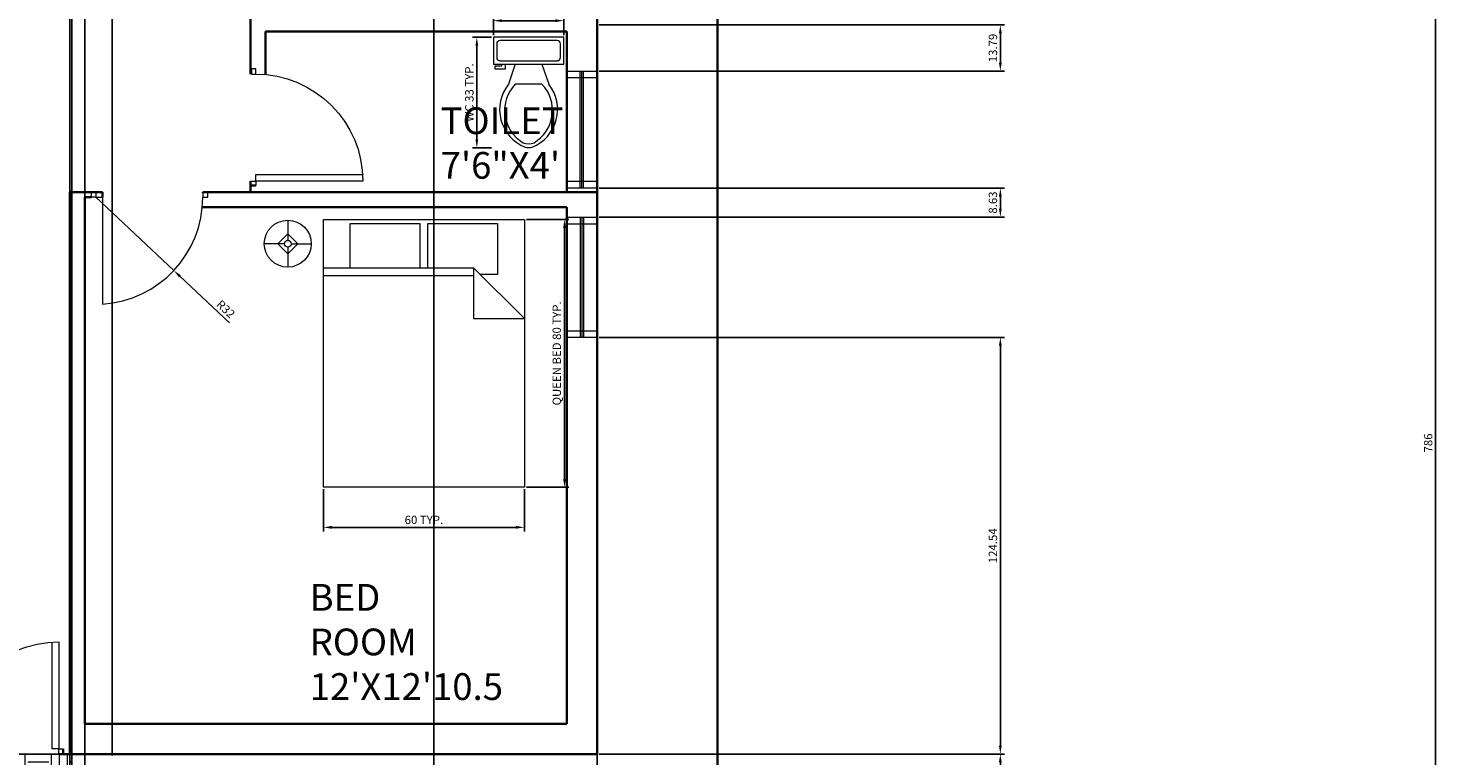
# Model space of a CAD drawing. Units: inches. Extents: x 204 to 942, y 1794 to 2670.
# Tile 5 of 6: x 521 to 942, y 2138 to 2355. Entities that reach past the tile are written whole.
import ezdxf

# ---------------------------------------------------------------- set-up
doc = ezdxf.new("R2010")
doc.units = ezdxf.units.IN
for name, color, linetype, lineweight in [('A-ANNO-DIMS', 2, 'Continuous', 18), ('A-AREA-IDEN', 7, 'Continuous', 18), ('A-DOOR', 3, 'Continuous', 18), ('A-FLOR-FIXT', 9, 'Continuous', 18), ('A-FLOR-OTLN', 7, 'Continuous', 25), ('A-FLOR-STRS', 7, 'Continuous', 25), ('A-FURN', 8, 'Continuous', 18), ('A-GLAZ', 4, 'Continuous', 18), ('A-WALL', 7, 'Continuous', 35), ('C-PROP', 7, 'Continuous', 35)]:
    doc.layers.add(name, color=color, linetype=linetype, lineweight=lineweight)
doc.layers.add('A-FLOR-PATT', color=251, linetype='Continuous', lineweight=13, true_color=0x636466)
doc.styles.get("Standard").update_dxf_attribs({"font": 'arial.ttf'})
doc.dimstyles.new('ISO-25', dxfattribs={"dimtxt": 2.5, "dimasz": 2.5, "dimexe": 1.25, "dimexo": 0.625, "dimtad": 1, "dimtxsty": 'Standard', "dimcen": 2.5, "dimadec": 0, "dimazin": 0, "dimtfac": 1, "dimtmove": 0, "dimatfit": 3, "dimfxl": 1, "dimarcsym": 0})

# ---------------------------------------------------------------- blocks, each defined once
blk = doc.blocks.new('Bed - Queen')
for p, q in [((0, -80.00003), (0, 0)), ((0, 0), (59.99999, 0)), ((59.99999, 0), (59.99999, -80.00003)), ((7.99999, -1.2), (28.79998, -1.2)), ((7.99999, -14.4), (7.99999, -1.2)), ((28.79998, -1.2), (28.79998, -14.4)), ((31.19999, -1.2), (51.99999, -1.2)), ((31.19999, -14.4), (31.19999, -1.2)), ((51.99999, -1.2), (51.99999, -16.4)), ((0, -14.4), (44.8, -14.4)), ((44.8, -16.8), (0, -16.8)), ((59.99999, -29.6), (44.8, -14.4)), ((44.8, -14.4), (44.8, -29.6)), ((51.99999, -16.4), (46.79936, -16.4)), ((44.8, -29.6), (59.99999, -29.6)), ((59.99999, -80.00003), (0, -80.00003))]:
    blk.add_line(p, q)
blk = doc.blocks.new('Lamp - Table')
for p, q in [((0, 7), (0, 1)), ((-1, 0), (-7, 0)), ((0, 3), (-3, 0)), ((-3, 0), (0, -3)), ((3, 0), (0, 3)), ((0, -3), (3, 0)), ((1, 0), (7, 0)), ((0, -1), (0, -7))]:
    blk.add_line(p, q)
for radius in [7, 1]:
    blk.add_circle((0, 0), radius)
blk = doc.blocks.new('Toilet - top')
for p, q in [((9.5, -6), (9.5, -2)), ((-8, -8.5), (-8, -8)), ((-7, -8), (-7, -9.5)), ((-4, -8), (-6, -14)), ((4, -8), (6, -14)), ((-10, -8.5), (-8, -8.5)), ((-10, -9.5), (-10, -8.5)), ((-7, -9.5), (-10, -9.5)), ((4, -14), (-4, -14))]:
    blk.add_line(p, q)
blk.add_lwpolyline([(10.5, -8), (10.5, 0), (-10.5, 0), (-10.5, -8)], close=True)
for points in [[(-9.5, -2), (-9.5, -6)], [(8.5, -1), (-8.5, -1)], [(-8.5, -7), (8.5, -7)]]:
    blk.add_lwpolyline(points)
for centre, radius, start, end in [((-8.62, -1.88), 0.884, 81.8699, 188.1301), ((8.62, -1.88), 0.884, 351.8699, 98.1301), ((-8.62, -6.12), 0.884, 171.8699, 278.1301), ((8.62, -6.12), 0.884, 261.8699, 8.1301), ((3.52, -21.58), 12.17, 141.4691, 247.9714), ((4.2, -21.82), 11.33, 136.3677, 238.9468), ((-3.52, -21.58), 12.17, 292.0284, 38.5307), ((-4.2, -21.82), 11.33, 301.053, 43.6321), ((0, -27.88), 4, 245.7318, 294.2682), ((0, -29), 4, 254.8605, 285.1395)]:
    blk.add_arc(centre, radius, start, end)
blk = doc.blocks.new('*D12')
at = {"layer": 'A-ANNO-DIMS', "color": 0, "lineweight": -2, "transparency": 16777216}
for p, q in [((727.37, 2624.26), (942.46, 2624.26)), ((941.21, 2621.76), (941.21, 1840.76)), ((727.37, 1838.26), (942.46, 1838.26))]:
    blk.add_line(p, q, dxfattribs=at)
at = {"layer": 'A-ANNO-DIMS', "color": 0, "transparency": 16777216}
for points in [[(940.79, 2621.76), (941.63, 2621.76), (941.21, 2624.26)], [(940.79, 1840.76), (941.63, 1840.76), (941.21, 1838.26)]]:
    blk.add_solid(points, dxfattribs=at)
at = {"layer": 'Defpoints', "color": 0, "transparency": 16777216}
for p in [(726.74, 2624.26), (726.74, 1838.26), (941.21, 1838.26)]:
    blk.add_point(p, dxfattribs=at)
at = {"layer": 'A-ANNO-DIMS', "color": 0, "transparency": 16777216, "insert": (939.31, 2231.26), "char_height": 2.5, "attachment_point": 5, "rotation": 90}
blk.add_mtext('786', dxfattribs=at)
blk = doc.blocks.new('WIN-36IN')
for p, q in [((0, 9), (36, 9)), ((0, 0), (0, 9)), ((2, 0), (2, 9)), ((34, 0), (34, 9)), ((36, 9), (36, 0)), ((0, 5), (36, 5)), ((0, 4.5), (36, 4.5)), ((0, 4), (36, 4)), ((36, 0), (0, 0)), ((0, 0), (2, 0)), ((36, 0), (34, 0))]:
    blk.add_line(p, q)
blk = doc.blocks.new('WIN-35IN')
for p, q in [((0, 0), (0, 35)), ((0, 35), (9, 35)), ((4, 0), (4, 35)), ((4.5, 0), (4.5, 35)), ((5, 0), (5, 35)), ((9, 35), (9, 0)), ((9, 35), (9, 33)), ((9, 33), (0, 33)), ((9, 2), (0, 2)), ((9, 0), (0, 0)), ((9, 0), (9, 2))]:
    blk.add_line(p, q)
blk = doc.blocks.new('DOOR-SWING-32IN')
for p, q in [((3.26, 1.55), (3.26, 33.49)), ((1.26, 1.55), (3.26, 1.55))]:
    blk.add_line(p, q)
blk.add_lwpolyline([(1.26, 33.55), (1.26, 1.55), (3.26, 1.55)])
for points in [[(1.26, 1.55), (0, 1.55), (0, 0), (1.26, 0)], [(33.26, 1.55), (34.79, 1.55), (34.79, 0.26), (33.26, 0.26)]]:
    blk.add_lwpolyline(points, close=True)
blk.add_arc((1.26, 1.55), 32, 0, 90)
blk = doc.blocks.new('*D22')
at = {"layer": 'A-ANNO-DIMS', "color": 0, "lineweight": -2, "transparency": 16777216}
for p, q in [((669.66, 2298.04), (682.29, 2298.04)), ((681.04, 2220.54), (681.04, 2295.54)), ((669.66, 2218.04), (682.29, 2218.04))]:
    blk.add_line(p, q, dxfattribs=at)
at = {"layer": 'A-ANNO-DIMS', "color": 0, "transparency": 16777216}
for points in [[(680.62, 2295.54), (681.46, 2295.54), (681.04, 2298.04)], [(680.62, 2220.54), (681.46, 2220.54), (681.04, 2218.04)]]:
    blk.add_solid(points, dxfattribs=at)
at = {"layer": 'Defpoints', "color": 0, "transparency": 16777216}
for p in [(669.04, 2298.04), (681.04, 2298.04), (669.04, 2218.04)]:
    blk.add_point(p, dxfattribs=at)
at = {"layer": 'A-ANNO-DIMS', "color": 0, "transparency": 16777216, "insert": (679.05, 2258.04), "char_height": 2.5, "attachment_point": 5, "rotation": 90}
blk.add_mtext('QUEEN BED 80 TYP.', dxfattribs=at)
blk = doc.blocks.new('*D23')
at = {"layer": 'A-ANNO-DIMS', "color": 0, "lineweight": -2, "transparency": 16777216}
for p, q in [((609.04, 2217.41), (609.04, 2204.79)), ((669.04, 2217.41), (669.04, 2204.79)), ((611.54, 2206.04), (666.54, 2206.04))]:
    blk.add_line(p, q, dxfattribs=at)
at = {"layer": 'A-ANNO-DIMS', "color": 0, "transparency": 16777216}
for points in [[(611.54, 2206.46), (611.54, 2205.62), (609.04, 2206.04)], [(666.54, 2206.46), (666.54, 2205.62), (669.04, 2206.04)]]:
    blk.add_solid(points, dxfattribs=at)
at = {"layer": 'Defpoints', "color": 0, "transparency": 16777216}
for p in [(609.04, 2218.04), (669.04, 2218.04), (669.04, 2206.04)]:
    blk.add_point(p, dxfattribs=at)
at = {"layer": 'A-ANNO-DIMS', "color": 0, "transparency": 16777216, "insert": (639.04, 2207.94), "char_height": 2.5, "attachment_point": 5}
blk.add_mtext('60 TYP.', dxfattribs=at)
blk = doc.blocks.new('*D26')
at = {"layer": 'A-ANNO-DIMS', "color": 0, "lineweight": -2, "transparency": 16777216}
for p, q in [((659.18, 2352.53), (653.6, 2352.53)), ((654.85, 2321.99), (654.85, 2350.03)), ((659.18, 2319.49), (653.6, 2319.49))]:
    blk.add_line(p, q, dxfattribs=at)
at = {"layer": 'A-ANNO-DIMS', "color": 0, "transparency": 16777216}
for points in [[(654.43, 2350.03), (655.26, 2350.03), (654.85, 2352.53)], [(654.43, 2321.99), (655.26, 2321.99), (654.85, 2319.49)]]:
    blk.add_solid(points, dxfattribs=at)
at = {"layer": 'Defpoints', "color": 0, "transparency": 16777216}
for p in [(654.85, 2352.53), (659.8, 2352.53), (659.8, 2319.49)]:
    blk.add_point(p, dxfattribs=at)
at = {"layer": 'A-ANNO-DIMS', "color": 0, "transparency": 16777216, "insert": (652.93, 2336.01), "char_height": 2.5, "attachment_point": 5, "rotation": 90}
blk.add_mtext('WC 33 TYP.', dxfattribs=at)
blk = doc.blocks.new('*D27')
at = {"layer": 'A-ANNO-DIMS', "color": 0, "lineweight": -2, "transparency": 16777216}
for p, q in [((659.8, 2353.16), (659.8, 2358.74)), ((662.3, 2357.49), (678.3, 2357.49)), ((680.8, 2353.16), (680.8, 2358.74))]:
    blk.add_line(p, q, dxfattribs=at)
at = {"layer": 'A-ANNO-DIMS', "color": 0, "transparency": 16777216}
for points in [[(662.3, 2357.91), (662.3, 2357.07), (659.8, 2357.49)], [(678.3, 2357.91), (678.3, 2357.07), (680.8, 2357.49)]]:
    blk.add_solid(points, dxfattribs=at)
at = {"layer": 'Defpoints', "color": 0, "transparency": 16777216}
for p in [(680.8, 2357.49), (659.8, 2352.53), (680.8, 2352.53)]:
    blk.add_point(p, dxfattribs=at)
at = {"layer": 'A-ANNO-DIMS', "color": 0, "transparency": 16777216, "insert": (670.3, 2359.37), "char_height": 2.5, "attachment_point": 5}
blk.add_mtext('21 TYP.', dxfattribs=at)
blk = doc.blocks.new('*D45')
at = {"layer": 'A-ANNO-DIMS', "color": 0, "lineweight": -2, "transparency": 16777216}
for p, q in [((691.37, 2138.26), (812.46, 2138.26)), ((811.21, 2016.68), (811.21, 2135.76)), ((691.37, 2014.18), (812.46, 2014.18))]:
    blk.add_line(p, q, dxfattribs=at)
at = {"layer": 'A-ANNO-DIMS', "color": 0, "transparency": 16777216}
for points in [[(810.79, 2135.76), (811.62, 2135.76), (811.21, 2138.26)], [(810.79, 2016.68), (811.62, 2016.68), (811.21, 2014.18)]]:
    blk.add_solid(points, dxfattribs=at)
at = {"layer": 'Defpoints', "color": 0, "transparency": 16777216}
for p in [(690.74, 2138.26), (811.21, 2138.26), (690.74, 2014.18)]:
    blk.add_point(p, dxfattribs=at)
at = {"layer": 'A-ANNO-DIMS', "color": 0, "transparency": 16777216, "insert": (809.31, 2076.22), "char_height": 2.5, "attachment_point": 5, "rotation": 90}
blk.add_mtext('124.08', dxfattribs=at)
blk = doc.blocks.new('*D47')
at = {"layer": 'A-ANNO-DIMS', "color": 0, "lineweight": -2, "transparency": 16777216}
for p, q in [((533.86, 2137.88), (533.86, 2668.11)), ((536.36, 2666.86), (543.38, 2666.86)), ((545.88, 2137.88), (545.88, 2668.11))]:
    blk.add_line(p, q, dxfattribs=at)
at = {"layer": 'A-ANNO-DIMS', "color": 0, "transparency": 16777216}
for points in [[(536.36, 2667.28), (536.36, 2666.44), (533.86, 2666.86)], [(543.38, 2667.28), (543.38, 2666.44), (545.88, 2666.86)]]:
    blk.add_solid(points, dxfattribs=at)
at = {"layer": 'Defpoints', "color": 0, "transparency": 16777216}
for p in [(545.88, 2666.86), (533.86, 2137.26), (545.88, 2137.26)]:
    blk.add_point(p, dxfattribs=at)
at = {"layer": 'A-ANNO-DIMS', "color": 0, "transparency": 16777216, "insert": (539.87, 2668.76), "char_height": 2.5, "attachment_point": 5}
blk.add_mtext('12.012', dxfattribs=at)
blk = doc.blocks.new('*D48')
at = {"layer": 'A-ANNO-DIMS', "color": 0, "lineweight": -2, "transparency": 16777216}
for p, q in [((641.98, 2014.8), (641.98, 2668.11)), ((644.48, 2666.86), (688.24, 2666.86)), ((690.74, 2014.8), (690.74, 2668.11))]:
    blk.add_line(p, q, dxfattribs=at)
at = {"layer": 'A-ANNO-DIMS', "color": 0, "transparency": 16777216}
for points in [[(644.48, 2667.28), (644.48, 2666.44), (641.98, 2666.86)], [(688.24, 2667.28), (688.24, 2666.44), (690.74, 2666.86)]]:
    blk.add_solid(points, dxfattribs=at)
at = {"layer": 'Defpoints', "color": 0, "transparency": 16777216}
for p in [(690.74, 2666.86), (641.98, 2014.18), (690.74, 2014.18)]:
    blk.add_point(p, dxfattribs=at)
at = {"layer": 'A-ANNO-DIMS', "color": 0, "transparency": 16777216, "insert": (666.36, 2668.76), "char_height": 2.5, "attachment_point": 5}
blk.add_mtext('48.77', dxfattribs=at)
blk = doc.blocks.new('*D50')
at = {"layer": 'A-ANNO-DIMS', "color": 0, "lineweight": -2, "transparency": 16777216}
for p, q in [((533.24, 2587.63), (533.24, 1794.41)), ((537.74, 2578.63), (537.74, 1794.41)), ((530.74, 1795.66), (528.24, 1795.66)), ((533.24, 1795.66), (537.74, 1795.66)), ((540.24, 1795.66), (548.67, 1795.66))]:
    blk.add_line(p, q, dxfattribs=at)
at = {"layer": 'A-ANNO-DIMS', "color": 0, "transparency": 16777216}
for points in [[(530.74, 1796.08), (530.74, 1795.24), (533.24, 1795.66)], [(540.24, 1796.08), (540.24, 1795.24), (537.74, 1795.66)]]:
    blk.add_solid(points, dxfattribs=at)
at = {"layer": 'Defpoints', "color": 0, "transparency": 16777216}
for p in [(533.24, 2588.26), (537.74, 2579.26), (537.74, 1795.66)]:
    blk.add_point(p, dxfattribs=at)
at = {"layer": 'A-ANNO-DIMS', "color": 0, "transparency": 16777216, "insert": (545.7, 1797.56), "char_height": 2.5, "attachment_point": 5}
blk.add_mtext('4.5', dxfattribs=at)
blk = doc.blocks.new('*D60')
at = {"layer": 'A-ANNO-DIMS', "color": 0, "lineweight": -2, "transparency": 16777216}
for p, q in [((691.38, 2262.8), (812.46, 2262.8)), ((811.21, 2140.76), (811.21, 2260.3)), ((691.37, 2138.26), (812.46, 2138.26))]:
    blk.add_line(p, q, dxfattribs=at)
at = {"layer": 'A-ANNO-DIMS', "color": 0, "transparency": 16777216}
for points in [[(810.79, 2260.3), (811.62, 2260.3), (811.21, 2262.8)], [(810.79, 2140.76), (811.62, 2140.76), (811.21, 2138.26)]]:
    blk.add_solid(points, dxfattribs=at)
at = {"layer": 'Defpoints', "color": 0, "transparency": 16777216}
for p in [(690.76, 2262.8), (811.21, 2262.8), (690.74, 2138.26)]:
    blk.add_point(p, dxfattribs=at)
at = {"layer": 'A-ANNO-DIMS', "color": 0, "transparency": 16777216, "insert": (809.31, 2200.53), "char_height": 2.5, "attachment_point": 5, "rotation": 90}
blk.add_mtext('124.54', dxfattribs=at)
blk = doc.blocks.new('*D61')
at = {"layer": 'A-ANNO-DIMS', "color": 0, "lineweight": -2, "transparency": 16777216}
for p, q in [((691.38, 2356.22), (812.46, 2356.22)), ((811.21, 2344.93), (811.21, 2353.72)), ((691.38, 2342.43), (812.46, 2342.43))]:
    blk.add_line(p, q, dxfattribs=at)
at = {"layer": 'A-ANNO-DIMS', "color": 0, "transparency": 16777216}
for points in [[(810.79, 2353.72), (811.62, 2353.72), (811.21, 2356.22)], [(810.79, 2344.93), (811.62, 2344.93), (811.21, 2342.43)]]:
    blk.add_solid(points, dxfattribs=at)
at = {"layer": 'Defpoints', "color": 0, "transparency": 16777216}
for p in [(690.76, 2356.22), (811.21, 2356.22), (690.75, 2342.43)]:
    blk.add_point(p, dxfattribs=at)
at = {"layer": 'A-ANNO-DIMS', "color": 0, "transparency": 16777216, "insert": (809.31, 2349.33), "char_height": 2.5, "attachment_point": 5, "rotation": 90}
blk.add_mtext('13.79', dxfattribs=at)
blk = doc.blocks.new('*D62')
at = {"layer": 'A-ANNO-DIMS', "color": 0, "lineweight": -2, "transparency": 16777216}
for p, q in [((691.38, 2307.43), (812.46, 2307.43)), ((811.21, 2301.3), (811.21, 2304.93)), ((691.38, 2298.8), (812.46, 2298.8))]:
    blk.add_line(p, q, dxfattribs=at)
at = {"layer": 'A-ANNO-DIMS', "color": 0, "transparency": 16777216}
for points in [[(810.79, 2304.93), (811.62, 2304.93), (811.21, 2307.43)], [(810.79, 2301.3), (811.62, 2301.3), (811.21, 2298.8)]]:
    blk.add_solid(points, dxfattribs=at)
at = {"layer": 'Defpoints', "color": 0, "transparency": 16777216}
for p in [(690.75, 2307.43), (811.21, 2307.43), (690.76, 2298.8)]:
    blk.add_point(p, dxfattribs=at)
at = {"layer": 'A-ANNO-DIMS', "color": 0, "transparency": 16777216, "insert": (809.31, 2303.12), "char_height": 2.5, "attachment_point": 5, "rotation": 90}
blk.add_mtext('8.63', dxfattribs=at)
blk = doc.blocks.new('*D63')
at = {"layer": 'A-ANNO-DIMS', "color": 0, "lineweight": -2, "transparency": 16777216}
for p, q in [((541.01, 2304.71), (564.33, 2282.8)), ((580.95, 2267.19), (566.15, 2281.09))]:
    blk.add_line(p, q, dxfattribs=at)
at = {"layer": 'A-ANNO-DIMS', "color": 0, "transparency": 16777216}
blk.add_solid([(566.44, 2281.39), (565.87, 2280.78), (564.33, 2282.8)], dxfattribs=at)
at = {"layer": 'Defpoints', "color": 0, "transparency": 16777216}
for p in [(541.01, 2304.71), (564.33, 2282.8)]:
    blk.add_point(p, dxfattribs=at)
at = {"layer": 'A-ANNO-DIMS', "color": 0, "transparency": 16777216, "insert": (579.63, 2271.04), "char_height": 2.5, "attachment_point": 5, "rotation": 316.7911}
blk.add_mtext('R32', dxfattribs=at)

msp = doc.modelspace()

# ---------------------------------------------------------------- hatches: boundary and pattern name
at = {"layer": 'A-FLOR-PATT'}
h = msp.add_hatch(dxfattribs=at)
h.set_pattern_fill('EARTH', color=256)
h.paths.add_polyline_path([(533.8633, 2137.2597), (533.8633, 2138.2597), (473.5284, 2138.2597), (473.5284, 2138.2472), (471.5284, 2138.2472), (437.5284, 2138.2472), (372.7443, 2138.2597), (336.7443, 2138.2597), (336.7443, 2014.1774), (533.8633, 2014.1774)])

# ---------------------------------------------------------------- linework, layer by layer
at = {"layer": 'A-DOOR'}
for p, q in [((541.0064, 2304.7082), (543.0064, 2304.7082)), ((543.0064, 2304.7082), (543.0064, 2272.7707))]:
    msp.add_line(p, q, dxfattribs=at)
for points in [[(541.0064, 2304.7082), (539.7443, 2304.7082), (539.7443, 2306.2597), (541.0064, 2306.2597)], [(573.0064, 2304.7082), (574.53, 2304.7082), (574.53, 2306.0038), (573.0064, 2306.0038)]]:
    msp.add_lwpolyline(points, close=True, dxfattribs=at)
msp.add_lwpolyline([(541.0064, 2304.7082), (543.0064, 2304.7082)], dxfattribs=at)
msp.add_arc((541.0064, 2304.7082), 32, 273.583322, 0, dxfattribs=at)
at = {"layer": 'A-FLOR-OTLN'}
msp.add_lwpolyline([(372.7443, 2588.2597), (690.7443, 2588.2597), (690.7443, 2138.2597), (372.7443, 2138.2597)], close=True, dxfattribs=at)
at = {"layer": 'A-FLOR-STRS'}
for p, q in [((533.8633, 2014.1774), (533.8633, 2138.2597)), ((641.9756, 2014.1774), (641.9756, 2138.2597)), ((690.7443, 2138.2597), (690.7443, 2014.1774))]:
    msp.add_line(p, q, dxfattribs=at)
at = {"layer": 'A-WALL'}
for p, q in [((690.7443, 2411.2597), (690.7443, 2330.2597)), ((587.2443, 2341.4841), (587.2443, 2358.7597)), ((681.7443, 2354.2597), (591.7443, 2354.2597)), ((591.7443, 2341.3856), (591.7443, 2354.2597)), ((681.7443, 2354.2597), (681.7443, 2306.2597)), ((690.7443, 2354.2597), (690.7443, 2301.7597)), ((533.2443, 2147.2597), (533.2443, 2306.2597)), ((537.7443, 2306.2597), (533.2443, 2306.2597)), ((537.7443, 2306.2597), (541.0064, 2306.2597)), ((537.7443, 2306.2597), (539.7443, 2306.2597)), ((541.0064, 2306.2597), (543.0064, 2306.2597)), ((543.0064, 2306.2597), (543.0064, 2304.7082)), ((573.0064, 2306.2597), (690.7443, 2306.2597)), ((573.0064, 2306.0038), (573.0064, 2306.2597)), ((587.2443, 2306.2597), (587.2443, 2309.5218)), ((587.2443, 2306.2597), (587.2443, 2308.2597)), ((587.2443, 2308.2597), (588.7958, 2308.2597)), ((681.7443, 2306.2597), (591.7443, 2306.2597)), ((537.7443, 2147.2597), (537.7443, 2304.7082)), ((539.7443, 2304.7082), (537.7443, 2304.7082)), ((537.7443, 2147.2597), (537.7443, 2301.7597)), ((572.8703, 2301.7597), (681.7443, 2301.7597)), ((681.7443, 2301.7597), (591.7443, 2301.7597)), ((681.7443, 2301.7597), (681.7443, 2147.2597)), ((690.7443, 2301.7597), (690.7443, 2138.2597)), ((533.2443, 2147.2597), (533.2443, 2138.2597)), ((681.7443, 2147.2597), (537.7443, 2147.2597)), ((529.9822, 2138.2597), (537.7443, 2138.2597)), ((531.2443, 2138.2597), (531.2443, 2139.8112)), ((533.2443, 2138.2597), (531.2443, 2138.2597)), ((690.7443, 2138.2597), (537.7443, 2138.2597))]:
    msp.add_line(p, q, dxfattribs=at)
at = {"layer": 'C-PROP'}
for p, q in [((726.7443, 2354.2597), (726.7443, 2301.7597)), ((726.7443, 2354.2597), (726.7443, 2301.7597)), ((726.7443, 2301.7597), (726.7443, 2138.2597))]:
    msp.add_line(p, q, dxfattribs=at)
msp.add_lwpolyline([(336.7443, 2102.2597), (336.7443, 2624.2597), (726.7443, 2624.2597), (726.7443, 2102.2597)], dxfattribs=at)

# ---------------------------------------------------------------- block references
at = {"layer": 'A-DOOR', "extrusion": (0, 0, -1), "zscale": -1, "rotation": 90.00000000000075}
msp.add_blockref('DOOR-SWING-32IN', (-587.2446, 2308.2594), dxfattribs=at)
at = {"layer": 'A-DOOR', "extrusion": (0, 0, -1), "zscale": -1}
msp.add_blockref('DOOR-SWING-32IN', (-531.2446, 2138.26), dxfattribs=at)
at = {"layer": 'A-FLOR-FIXT'}
msp.add_blockref('Toilet - top', (670.3042, 2352.5328), dxfattribs=at)
at = {"layer": 'A-FURN'}
for name, p in [('Lamp - Table', (598.374, 2290.8143)), ('Bed - Queen', (609.04, 2298.0388))]:
    msp.add_blockref(name, p, dxfattribs=at)
at = {"layer": 'A-GLAZ'}
msp.add_blockref('WIN-35IN', (681.7515, 2307.4314), dxfattribs=at)
at = {"layer": 'A-GLAZ', "rotation": 269.9999999999977}
msp.add_blockref('WIN-36IN', (681.7555, 2298.8003), dxfattribs=at)

# ---------------------------------------------------------------- texts
at = {"layer": 'A-AREA-IDEN', "char_height": 2.5, "attachment_point": 1}
for s, insert in [('{\\H3.2x;TOILET\\P7\'6"X4\' }', (644.0399, 2331.587)), ("{\\H3.2x;BED ROOM\\P12'X12'10.5 }", (604.9109, 2189.1145))]:
    msp.add_mtext_dynamic_manual_height_columns(s, width=46.676204, gutter_width=12.5, heights=[0], dxfattribs=dict(at, insert=insert))

# ---------------------------------------------------------------- dimensions: what is measured, and where the dimension line sits
at = {"layer": 'A-ANNO-DIMS'}
for base, p1, p2, override, picture, middle in [((545.8757, 2666.8597), (533.8633, 2137.2597), (545.8757, 2137.2597), {"dimdec": 3, "dimlfac": 1, "dimrnd": 0, "dimzin": 0, "dimdsep": 46, "dimlunit": 2}, '*D47', (539.8695, 2668.7611)), ((690.7443, 2666.8597), (641.9756, 2014.1774), (690.7443, 2014.1774), {"dimdec": 2, "dimlfac": 1, "dimrnd": 0, "dimzin": 0, "dimdsep": 46, "dimlunit": 2}, '*D48', (666.3599, 2668.7611)), ((537.7443, 1795.6597), (533.2443, 2588.2597), (537.7443, 2579.2597), {"dimdec": 1, "dimlfac": 1, "dimrnd": 0, "dimzin": 0, "dimdsep": 46, "dimlunit": 2}, '*D50', (545.7047, 1797.556))]:
    dim = msp.add_linear_dim(base=base, p1=p1, p2=p2, dimstyle='ISO-25', override=override, dxfattribs=at)
    dim.commit()
    dim.dimension.update_dxf_attribs({"geometry": picture, "text_midpoint": middle})
for base, p1, p2, override, picture, middle in [((941.2084, 1838.2597), (726.7443, 2624.2597), (726.7443, 1838.2597), {"dimclrd": 0, "dimclre": 0, "dimclrt": 0}, '*D12', (939.307, 2231.2597)), ((811.2079, 2356.22), (690.7515, 2342.4314), (690.756, 2356.22), {"dimdec": 2, "dimlfac": 1, "dimrnd": 0, "dimzin": 0, "dimdsep": 46, "dimlunit": 2}, '*D61', (809.3056, 2349.3257)), ((811.2079, 2307.4314), (690.7557, 2298.8008), (690.7515, 2307.4314), {"dimdec": 2, "dimlfac": 1, "dimrnd": 0, "dimzin": 0, "dimdsep": 46, "dimlunit": 2}, '*D62', (809.3056, 2303.1161)), ((811.2079, 2262.8008), (690.7443, 2138.2597), (690.7557, 2262.8008), {"dimdec": 2, "dimlfac": 1, "dimrnd": 0, "dimzin": 0, "dimdsep": 46, "dimlunit": 2}, '*D60', (809.3064, 2200.5302)), ((811.2079, 2138.2597), (690.7443, 2014.1774), (690.7443, 2138.2597), {"dimdec": 2, "dimlfac": 1, "dimrnd": 0, "dimzin": 0, "dimdsep": 46, "dimlunit": 2}, '*D45', (809.3064, 2076.2185))]:
    dim = msp.add_linear_dim(base=base, p1=p1, p2=p2, angle=90, dimstyle='ISO-25', override=override, dxfattribs=at)
    dim.commit()
    dim.dimension.update_dxf_attribs({"geometry": picture, "text_midpoint": middle})
for base, p1, p2, picture, middle in [((680.8042, 2357.4898), (659.8042, 2352.5328), (680.8042, 2352.5328), '*D27', (670.3042, 2359.3707)), ((669.04, 2206.0387), (609.04, 2218.0387), (669.04, 2218.0387), '*D23', (639.04, 2207.9402))]:
    dim = msp.add_linear_dim(base=base, p1=p1, p2=p2, text='<> TYP.', dimstyle='ISO-25', override={"dimdec": 0, "dimlfac": 1, "dimrnd": 0, "dimzin": 0, "dimdsep": 46, "dimlunit": 2}, dxfattribs=at)
    dim.commit()
    dim.dimension.update_dxf_attribs({"geometry": picture, "text_midpoint": middle})
for base, p1, p2, text, picture, middle in [((654.8473, 2352.5328), (659.8042, 2319.4866), (659.8042, 2352.5328), 'WC <> TYP.', '*D26', (652.9288, 2336.0097)), ((681.04, 2298.0388), (669.04, 2218.0387), (669.04, 2298.0388), 'QUEEN BED <> TYP.', '*D22', (679.0456, 2258.0387))]:
    dim = msp.add_linear_dim(base=base, p1=p1, p2=p2, angle=90, text=text, dimstyle='ISO-25', override={"dimdec": 0, "dimlfac": 1, "dimrnd": 0, "dimzin": 0, "dimdsep": 46, "dimlunit": 2}, dxfattribs=at)
    dim.commit()
    dim.dimension.update_dxf_attribs({"geometry": picture, "text_midpoint": middle})
dim = msp.add_radius_dim(center=(541.0064, 2304.7082), mpoint=(564.33, 2282.799), dimstyle='ISO-25', override={"dimdec": 0, "dimlfac": 1, "dimrnd": 0, "dimzin": 0, "dimdsep": 46, "dimlunit": 2}, dxfattribs=at)
dim.commit()
dim.dimension.update_dxf_attribs({"geometry": '*D63', "text_midpoint": (578.3241, 2269.6535), "dimtype": 164})

doc.saveas('drawing.dxf')
